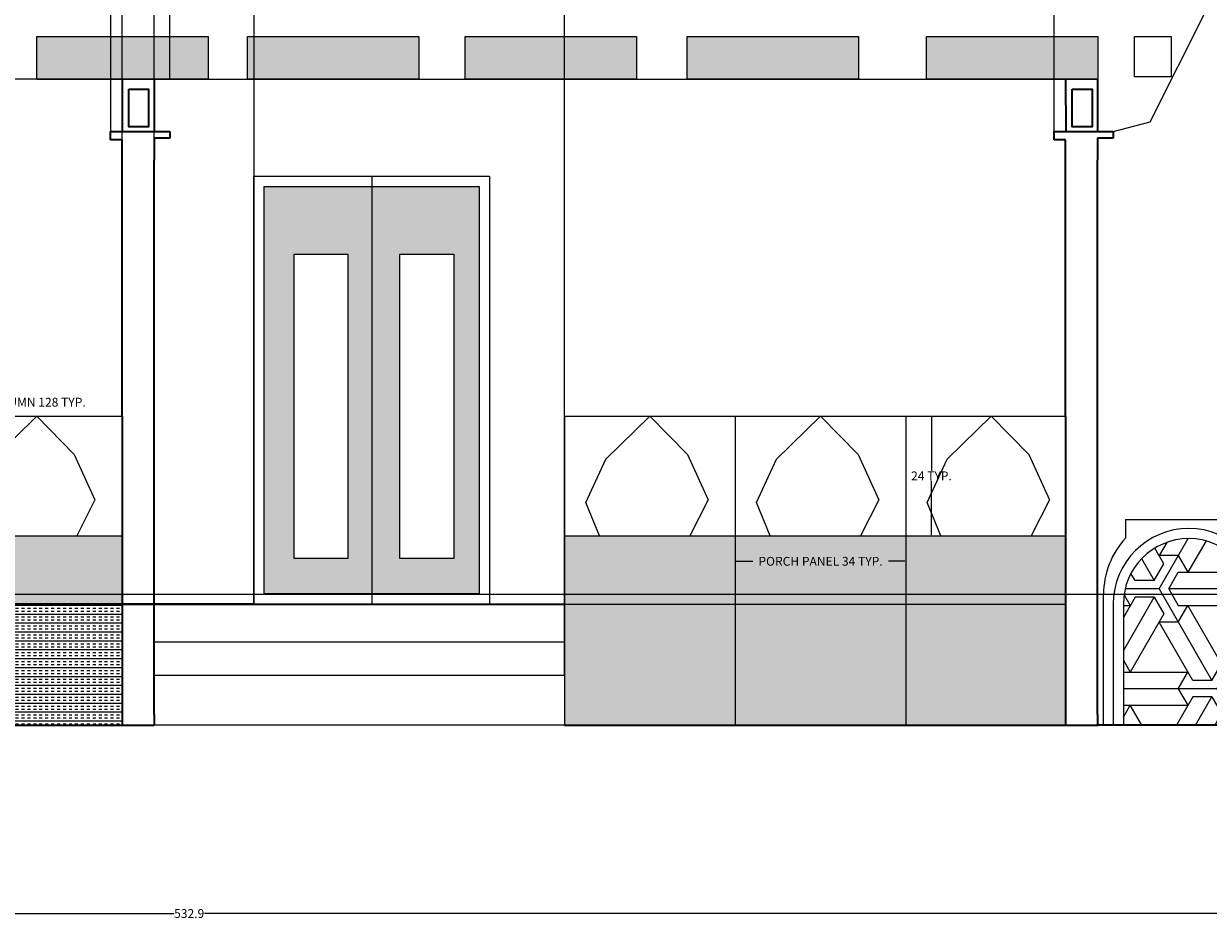
# Model space of a CAD drawing. Units: inches. Extents: x -17 to 741, y 7 to 490.
# Tile 3 of 8: x 254 to 489, y 14 to 191. Entities that reach past the tile are written whole.
import ezdxf

# ---------------------------------------------------------------- set-up
doc = ezdxf.new("R2010")
doc.units = ezdxf.units.IN
doc.header["$MEASUREMENT"] = 0
for name, color, linetype, lineweight in [('A-ANNO-DIMS', 2, 'Continuous', 18), ('A-COLS', 1, 'Continuous', 35), ('A-DOOR', 3, 'Continuous', 25), ('A-ELEV-PATT', 252, 'Continuous', 13), ('A-FLOR-RAIL', 7, 'Continuous', 25), ('A-FLOR-STRS', 7, 'Continuous', 25), ('A-ROOF-CNPE', 7, 'Continuous', 25), ('A-WALL', 7, 'Continuous', 35), ('A-WALL-PATT', 8, 'Continuous', 13), ('A-WALL-SCRN', 7, 'Continuous', 25)]:
    doc.layers.add(name, color=color, linetype=linetype, lineweight=lineweight)
doc.styles.get("Standard").update_dxf_attribs({"font": 'arial.ttf'})
doc.dimstyles.get("Standard").update_dxf_attribs({"dimtxt": 1.75, "dimasz": 0.18, "dimexe": 0.18, "dimexo": 0.0625, "dimgap": 0.09, "dimtad": 0, "dimtih": 1, "dimtoh": 1, "dimdec": 4, "dimzin": 0, "dimdsep": 46, "dimlunit": 4, "dimtxsty": 'Standard', "dimcen": 0.09, "dimadec": 0, "dimazin": 0, "dimtfac": 1, "dimtdec": 4, "dimtofl": 0, "dimtmove": 0, "dimatfit": 3, "dimfxl": 1, "dimtolj": 1, "dimtzin": 0, "dimarcsym": 0})

# ---------------------------------------------------------------- blocks, each defined once
blk = doc.blocks.new('SCREEN-ARCH-END-BAY')
for p, q in [((4.33, 40.71), (4.33, 37.01)), ((4.33, 40.71), (31.23, 40.71)), ((31.23, 40.71), (31.23, 37.52)), ((31.23, 37.52), (33.14, 37.52)), ((33.14, 37.52), (33.61, 37.52)), ((33.61, 37.52), (33.61, 0)), ((36.63, 37.52), (36.63, 0)), ((0, 0), (0, 25.9))]:
    blk.add_line(p, q)
for points in [[(31.83, 0), (31.83, 24, 1), (1.92, 24), (1.92, 0)], [(29.83, 0), (29.83, 24, 1), (3.92, 24), (3.92, 0)]]:
    blk.add_lwpolyline(points, format="xyb")
for centre, radius, start in [((35.12, 37.52), 1.51, 0), ((16.41, 25.9), 16.41, 137.3839)]:
    blk.add_arc(centre, radius, start, 180)
blk = doc.blocks.new('COL-PORCH-CAPPED')
for p, q in [((2.37, 117.52), (2.32, 127.86)), ((8.64, 117.52), (8.64, 127.86)), ((0, 115.82), (0, 117.52)), ((0, 117.52), (11.68, 117.52)), ((11.68, 117.52), (11.68, 116.2)), ((2.25, 115.82), (0, 115.82)), ((2.25, 109.13), (2.25, 115.82)), ((11.68, 116.2), (8.61, 116.2)), ((8.61, 116.2), (8.61, 111.83)), ((8.61, 2.12), (8.61, 111.83)), ((2.25, 61.18), (2.25, 109.13)), ((2.25, 61.18), (2.25, 0)), ((8.61, 2.12), (8.61, 0))]:
    blk.add_line(p, q)
blk.add_lwpolyline([(3.57, 125.89), (7.5, 125.89), (7.5, 118.41), (3.57, 118.41)], close=True)
blk = doc.blocks.new('DOOR-PAIR-FRAME')
blk.add_line((23.28, 84.63), (23.28, 0))
for points in [[(0, 84.63), (46.56, 84.63), (46.56, 0), (0, 0)], [(2, 82.63), (44.56, 82.63), (44.56, 2), (2, 2)]]:
    blk.add_lwpolyline(points, close=True)
blk = doc.blocks.new('PORCH-POINTED-PANEL')
for p, q in [((0, 23.66), (33.75, 23.66)), ((0, 0), (33.75, 0))]:
    blk.add_line(p, q)
blk.add_lwpolyline([(6.92, 0), (4.23, 6.56), (8.17, 15.14), (16.88, 23.66), (24.3, 16.07), (28.38, 7.1), (24.8, 0)])
blk = doc.blocks.new('*D17')
at = {"layer": 'A-ANNO-DIMS', "color": 0, "lineweight": -2, "transparency": 16777216}
for p, q in [((394.98, 89.46), (394.98, 84.28)), ((428.73, 89.46), (428.73, 84.28)), ((395.16, 84.46), (398.44, 84.46)), ((428.55, 84.46), (425.26, 84.46))]:
    blk.add_line(p, q, dxfattribs=at)
at = {"layer": 'A-ANNO-DIMS', "color": 0, "transparency": 16777216}
for points in [[(395.16, 84.49), (395.16, 84.43), (394.98, 84.46)], [(428.55, 84.49), (428.55, 84.43), (428.73, 84.46)]]:
    blk.add_solid(points, dxfattribs=at)
at = {"layer": 'Defpoints', "color": 0, "transparency": 16777216}
for p in [(394.98, 89.53), (428.73, 89.53), (428.73, 84.46)]:
    blk.add_point(p, dxfattribs=at)
at = {"layer": 'A-ANNO-DIMS', "color": 0, "transparency": 16777216, "insert": (411.85, 84.46), "char_height": 1.75, "attachment_point": 5}
blk.add_mtext('\\A1;PORCH PANEL 34 TYP.', dxfattribs=at)
blk = doc.blocks.new('*D18')
at = {"layer": 'A-ANNO-DIMS', "color": 0, "lineweight": -2, "transparency": 16777216}
for p, q in [((428.79, 113.19), (433.97, 113.19)), ((433.79, 113.01), (433.79, 102.33)), ((433.79, 89.71), (433.79, 100.39)), ((428.79, 89.53), (433.97, 89.53))]:
    blk.add_line(p, q, dxfattribs=at)
at = {"layer": 'A-ANNO-DIMS', "color": 0, "transparency": 16777216}
for points in [[(433.76, 113.01), (433.82, 113.01), (433.79, 113.19)], [(433.76, 89.71), (433.82, 89.71), (433.79, 89.53)]]:
    blk.add_solid(points, dxfattribs=at)
at = {"layer": 'Defpoints', "color": 0, "transparency": 16777216}
for p in [(428.73, 113.19), (433.79, 113.19), (428.73, 89.53)]:
    blk.add_point(p, dxfattribs=at)
at = {"layer": 'A-ANNO-DIMS', "color": 0, "transparency": 16777216, "insert": (433.79, 101.36), "char_height": 1.75, "attachment_point": 5}
blk.add_mtext('\\A1;24 TYP.', dxfattribs=at)
blk = doc.blocks.new('*D27')
at = {"layer": 'A-ANNO-DIMS', "color": 0, "lineweight": -2, "transparency": 16777216}
for p, q in [((271.37, 179.87), (252.08, 179.87)), ((252.26, 179.69), (252.26, 116.93)), ((252.26, 52.19), (252.26, 114.94)), ((271.37, 52.01), (252.08, 52.01))]:
    blk.add_line(p, q, dxfattribs=at)
at = {"layer": 'A-ANNO-DIMS', "color": 0, "transparency": 16777216}
for points in [[(252.23, 179.69), (252.29, 179.69), (252.26, 179.87)], [(252.23, 52.19), (252.29, 52.19), (252.26, 52.01)]]:
    blk.add_solid(points, dxfattribs=at)
at = {"layer": 'Defpoints', "color": 0, "transparency": 16777216}
for p in [(252.26, 179.87), (271.44, 179.87), (271.44, 52.01)]:
    blk.add_point(p, dxfattribs=at)
at = {"layer": 'A-ANNO-DIMS', "color": 0, "transparency": 16777216, "insert": (252.26, 115.94), "char_height": 1.75, "attachment_point": 5}
blk.add_mtext('\\A1;PORCH COLUMN 128 TYP.', dxfattribs=at)
blk = doc.blocks.new('*D28')
at = {"layer": 'A-ANNO-DIMS', "color": 0, "lineweight": -2, "transparency": 16777216}
for p, q in [((271.44, 179.93), (271.44, 199.23)), ((283.11, 179.93), (283.11, 199.23)), ((271.62, 199.05), (273.01, 199.05)), ((282.93, 199.05), (281.54, 199.05))]:
    blk.add_line(p, q, dxfattribs=at)
at = {"layer": 'A-ANNO-DIMS', "color": 0, "transparency": 16777216}
for points in [[(271.62, 199.08), (271.62, 199.02), (271.44, 199.05)], [(282.93, 199.08), (282.93, 199.02), (283.11, 199.05)]]:
    blk.add_solid(points, dxfattribs=at)
at = {"layer": 'Defpoints', "color": 0, "transparency": 16777216}
for p in [(283.11, 199.05), (271.44, 179.87), (283.11, 179.87)]:
    blk.add_point(p, dxfattribs=at)
at = {"layer": 'A-ANNO-DIMS', "color": 0, "transparency": 16777216, "insert": (277.28, 199.05), "char_height": 1.75, "attachment_point": 5}
blk.add_mtext('\\A1;12 TYP.', dxfattribs=at)
blk = doc.blocks.new('*D37')
at = {"layer": 'A-ANNO-DIMS', "color": 0, "lineweight": -2, "transparency": 16777216}
for p, q in [((20.52, 396.95), (20.52, 14.58)), ((553.43, 51.95), (553.43, 14.58)), ((20.7, 14.76), (283.93, 14.76)), ((553.25, 14.76), (290.02, 14.76))]:
    blk.add_line(p, q, dxfattribs=at)
at = {"layer": 'A-ANNO-DIMS', "color": 0, "transparency": 16777216}
for points in [[(20.7, 14.79), (20.7, 14.73), (20.52, 14.76)], [(553.25, 14.79), (553.25, 14.73), (553.43, 14.76)]]:
    blk.add_solid(points, dxfattribs=at)
at = {"layer": 'Defpoints', "color": 0, "transparency": 16777216}
for p in [(20.52, 397.01), (553.43, 52.01), (553.43, 14.76)]:
    blk.add_point(p, dxfattribs=at)
at = {"layer": 'A-ANNO-DIMS', "color": 0, "transparency": 16777216, "insert": (286.97, 14.76), "char_height": 1.75, "attachment_point": 5}
blk.add_mtext('\\A1;532.9', dxfattribs=at)
blk = doc.blocks.new('*D38')
at = {"layer": 'A-ANNO-DIMS', "color": 0, "lineweight": -2, "transparency": 16777216}
for p, q in [((341.83, 454.57), (723.06, 454.57)), ((722.88, 454.39), (722.88, 254.27)), ((722.88, 52.19), (722.88, 252.31)), ((553.49, 52.01), (723.06, 52.01))]:
    blk.add_line(p, q, dxfattribs=at)
at = {"layer": 'A-ANNO-DIMS', "color": 0, "transparency": 16777216}
for points in [[(722.85, 454.39), (722.91, 454.39), (722.88, 454.57)], [(722.85, 52.19), (722.91, 52.19), (722.88, 52.01)]]:
    blk.add_solid(points, dxfattribs=at)
at = {"layer": 'Defpoints', "color": 0, "transparency": 16777216}
for p in [(341.77, 454.57), (722.88, 454.57), (553.43, 52.01)]:
    blk.add_point(p, dxfattribs=at)
at = {"layer": 'A-ANNO-DIMS', "color": 0, "transparency": 16777216, "insert": (722.88, 253.29), "char_height": 1.75, "attachment_point": 5}
blk.add_mtext('\\A1;402.6', dxfattribs=at)
blk = doc.blocks.new('*D52')
at = {"layer": 'A-ANNO-DIMS', "color": 0, "lineweight": -2, "transparency": 16777216}
for p, q in [((239.94, 113.25), (239.94, 488.55)), ((240.12, 488.37), (253.76, 488.37)), ((273.51, 488.37), (259.86, 488.37)), ((273.69, 113.25), (273.69, 488.55))]:
    blk.add_line(p, q, dxfattribs=at)
at = {"layer": 'A-ANNO-DIMS', "color": 0, "transparency": 16777216}
for points in [[(240.12, 488.4), (240.12, 488.34), (239.94, 488.37)], [(273.51, 488.4), (273.51, 488.34), (273.69, 488.37)]]:
    blk.add_solid(points, dxfattribs=at)
at = {"layer": 'Defpoints', "color": 0, "transparency": 16777216}
for p in [(273.69, 488.37), (239.94, 113.19), (273.69, 113.19)]:
    blk.add_point(p, dxfattribs=at)
at = {"layer": 'A-ANNO-DIMS', "color": 0, "transparency": 16777216, "insert": (256.81, 488.37), "char_height": 1.75, "attachment_point": 5}
blk.add_mtext('\\A1;33.75', dxfattribs=at)
blk = doc.blocks.new('*D53')
at = {"layer": 'A-ANNO-DIMS', "color": 0, "lineweight": -2, "transparency": 16777216}
for p, q in [((271.44, 167.89), (271.44, 488.55)), ((271.62, 488.37), (361.78, 488.37)), ((457.87, 488.37), (367.7, 488.37)), ((458.05, 167.89), (458.05, 488.55))]:
    blk.add_line(p, q, dxfattribs=at)
at = {"layer": 'A-ANNO-DIMS', "color": 0, "transparency": 16777216}
for points in [[(271.62, 488.4), (271.62, 488.34), (271.44, 488.37)], [(457.87, 488.4), (457.87, 488.34), (458.05, 488.37)]]:
    blk.add_solid(points, dxfattribs=at)
at = {"layer": 'Defpoints', "color": 0, "transparency": 16777216}
for p in [(458.05, 488.37), (271.44, 167.83), (458.05, 167.83)]:
    blk.add_point(p, dxfattribs=at)
at = {"layer": 'A-ANNO-DIMS', "color": 0, "transparency": 16777216, "insert": (364.74, 488.37), "char_height": 1.75, "attachment_point": 5}
blk.add_mtext('\\A1;186.6', dxfattribs=at)
blk = doc.blocks.new('*D54')
at = {"layer": 'A-ANNO-DIMS', "color": 0, "lineweight": -2, "transparency": 16777216}
for p, q in [((458.05, 167.89), (458.05, 488.55)), ((458.23, 488.37), (502.69, 488.37)), ((553.25, 488.37), (508.78, 488.37)), ((553.43, 52.07), (553.43, 488.55))]:
    blk.add_line(p, q, dxfattribs=at)
at = {"layer": 'A-ANNO-DIMS', "color": 0, "transparency": 16777216}
for points in [[(458.23, 488.4), (458.23, 488.34), (458.05, 488.37)], [(553.25, 488.4), (553.25, 488.34), (553.43, 488.37)]]:
    blk.add_solid(points, dxfattribs=at)
at = {"layer": 'Defpoints', "color": 0, "transparency": 16777216}
for p in [(553.43, 488.37), (458.05, 167.83), (553.43, 52.01)]:
    blk.add_point(p, dxfattribs=at)
at = {"layer": 'A-ANNO-DIMS', "color": 0, "transparency": 16777216, "insert": (505.74, 488.37), "char_height": 1.75, "attachment_point": 5}
blk.add_mtext('\\A1;95.38', dxfattribs=at)
blk = doc.blocks.new('*D60')
at = {"layer": 'A-ANNO-DIMS', "color": 0, "lineweight": -2, "transparency": 16777216}
for p, q in [((280.05, 68.56), (280.05, 488.55)), ((280.23, 488.37), (286.96, 488.37)), ((299.61, 488.37), (292.87, 488.37)), ((299.79, 76.07), (299.79, 488.55))]:
    blk.add_line(p, q, dxfattribs=at)
at = {"layer": 'A-ANNO-DIMS', "color": 0, "transparency": 16777216}
for points in [[(280.23, 488.4), (280.23, 488.34), (280.05, 488.37)], [(299.61, 488.4), (299.61, 488.34), (299.79, 488.37)]]:
    blk.add_solid(points, dxfattribs=at)
at = {"layer": 'Defpoints', "color": 0, "transparency": 16777216}
for p in [(299.79, 488.37), (299.79, 76.01), (280.05, 68.49)]:
    blk.add_point(p, dxfattribs=at)
at = {"layer": 'A-ANNO-DIMS', "color": 0, "transparency": 16777216, "insert": (289.92, 488.37), "char_height": 1.75, "attachment_point": 5}
blk.add_mtext('\\A1;19.74', dxfattribs=at)
blk = doc.blocks.new('*D61')
at = {"layer": 'A-ANNO-DIMS', "color": 0, "lineweight": -2, "transparency": 16777216}
for p, q in [((225.78, 99.68), (-13.46, 99.68)), ((-13.28, 99.5), (-13.28, 88.83)), ((-13.28, 76.19), (-13.28, 86.86)), ((299.72, 76.01), (-13.46, 76.01))]:
    blk.add_line(p, q, dxfattribs=at)
at = {"layer": 'A-ANNO-DIMS', "color": 0, "transparency": 16777216}
for points in [[(-13.31, 99.5), (-13.25, 99.5), (-13.28, 99.68)], [(-13.31, 76.19), (-13.25, 76.19), (-13.28, 76.01)]]:
    blk.add_solid(points, dxfattribs=at)
at = {"layer": 'Defpoints', "color": 0, "transparency": 16777216}
for p in [(225.85, 99.68), (-13.28, 76.01), (299.79, 76.01)]:
    blk.add_point(p, dxfattribs=at)
at = {"layer": 'A-ANNO-DIMS', "color": 0, "transparency": 16777216, "insert": (-13.28, 87.85), "char_height": 1.75, "attachment_point": 5}
blk.add_mtext('\\A1;23.677', dxfattribs=at)
blk = doc.blocks.new('*D64')
at = {"layer": 'A-ANNO-DIMS', "color": 0, "lineweight": -2, "transparency": 16777216}
for p, q in [((516.74, 77.91), (-13.46, 77.91)), ((-13.28, 77.73), (-13.28, 65.94)), ((-13.28, 52.19), (-13.28, 63.98)), ((516.74, 52.01), (-13.46, 52.01))]:
    blk.add_line(p, q, dxfattribs=at)
at = {"layer": 'A-ANNO-DIMS', "color": 0, "transparency": 16777216}
for points in [[(-13.31, 77.73), (-13.25, 77.73), (-13.28, 77.91)], [(-13.31, 52.19), (-13.25, 52.19), (-13.28, 52.01)]]:
    blk.add_solid(points, dxfattribs=at)
at = {"layer": 'Defpoints', "color": 0, "transparency": 16777216}
for p in [(-13.28, 77.91), (516.8, 77.91), (516.8, 52.01)]:
    blk.add_point(p, dxfattribs=at)
at = {"layer": 'A-ANNO-DIMS', "color": 0, "transparency": 16777216, "insert": (-13.28, 64.96), "char_height": 1.75, "attachment_point": 5}
blk.add_mtext('\\A1;25.9', dxfattribs=at)
blk = doc.blocks.new('*D68')
at = {"layer": 'A-ANNO-DIMS', "color": 0, "lineweight": -2, "transparency": 16777216}
for p, q in [((280.05, 61.98), (280.05, 488.55)), ((280.23, 488.37), (317.59, 488.37)), ((361.04, 488.37), (323.68, 488.37)), ((361.22, 61.98), (361.22, 488.55))]:
    blk.add_line(p, q, dxfattribs=at)
at = {"layer": 'A-ANNO-DIMS', "color": 0, "transparency": 16777216}
for points in [[(280.23, 488.4), (280.23, 488.34), (280.05, 488.37)], [(361.04, 488.4), (361.04, 488.34), (361.22, 488.37)]]:
    blk.add_solid(points, dxfattribs=at)
at = {"layer": 'Defpoints', "color": 0, "transparency": 16777216}
for p in [(361.22, 488.37), (280.05, 61.91), (361.22, 61.91)]:
    blk.add_point(p, dxfattribs=at)
at = {"layer": 'A-ANNO-DIMS', "color": 0, "transparency": 16777216, "insert": (320.64, 488.37), "char_height": 1.75, "attachment_point": 5}
blk.add_mtext('\\A1;81.18', dxfattribs=at)

msp = doc.modelspace()

# ---------------------------------------------------------------- hatches: boundary and pattern name
at = {"layer": 'A-ELEV-PATT'}
h = msp.add_hatch(dxfattribs=at)
h.set_pattern_fill('STARS', color=256, scale=19)
h.paths.add_polyline_path([(204.6793, 330.2905), (174.1219, 330.2905), (174.1219, 324.7204), (204.6793, 324.7204)])
h.paths.add_polyline_path([(238.7618, 330.6251), (208.2044, 330.6251), (208.2044, 325.055), (238.7618, 325.055)])
h.paths.add_polyline_path([(316.4391, 354.2167), (282.5434, 354.2167), (282.5434, 345.7496), (316.4391, 345.7496)])
h.paths.add_polyline_path([(360.3395, 354.2167), (326.4438, 354.2167), (326.4438, 345.7496), (360.3395, 345.7496)])
h.paths.add_polyline_path([(407.6938, 354.2167), (373.7981, 354.2167), (373.7981, 345.7496), (407.6938, 345.7496)])
h.paths.add_polyline_path([(290.7055, 188.3373), (256.8098, 188.3373), (256.8098, 179.8702), (290.7055, 179.8702)])
h.paths.add_polyline_path([(332.372, 188.3373), (298.4763, 188.3373), (298.4763, 179.8702), (332.372, 179.8702)])
h.paths.add_polyline_path([(375.4339, 188.3373), (341.5382, 188.3373), (341.5382, 179.8702), (375.4339, 179.8702)])
h.paths.add_polyline_path([(419.3343, 188.3373), (385.4386, 188.3373), (385.4386, 179.8702), (419.3343, 179.8702)])
h.paths.add_polyline_path([(466.6886, 188.3373), (432.7929, 188.3373), (432.7929, 179.8702), (466.6886, 179.8702)])
h = msp.add_hatch(color=256, dxfattribs=at)
h.dxf.hatch_style = 1
h.paths.add_polyline_path([(323.0665, 158.6389), (301.7867, 158.6389), (301.7867, 78.0082), (323.0665, 78.0082)])
h.paths.add_polyline_path([(318.3825, 145.2592), (318.3825, 85.0354), (307.7462, 85.0354), (307.7462, 145.2592)], flags=16)
h.paths.add_polyline_path([(344.3462, 158.6389), (323.0665, 158.6389), (323.0665, 78.0082), (344.3462, 78.0082)])
h.paths.add_polyline_path([(339.3004, 145.2592), (339.3004, 85.0354), (328.6642, 85.0354), (328.6642, 145.2592)], flags=16)
h.paths.add_polyline_path([(192.7233, 151.6028), (190.2672, 151.6028), (190.2672, 142.0361), (192.7233, 142.0361)])
h.paths.add_polyline_path([(192.7233, 141.0361), (190.2672, 141.0361), (190.2672, 135.6738), (192.7233, 135.6738)])
h.paths.add_polyline_path([(192.7233, 142.0361), (190.2672, 142.0361), (190.2672, 141.0361), (192.7233, 141.0361)])
h.paths.add_polyline_path([(209.3698, 142.0361), (192.7233, 142.0361), (192.7233, 141.0361), (209.3698, 141.0361)])
h.paths.add_polyline_path([(190.2672, 142.0361), (183.5379, 142.0361), (183.5379, 141.0361), (190.2672, 141.0361)])
h.paths.add_polyline_path([(190.2672, 135.6738), (183.5379, 135.6738), (183.5379, 134.6738), (190.2672, 134.6738)])
h.paths.add_polyline_path([(192.7233, 135.6738), (190.2672, 135.6738), (190.2672, 134.6738), (192.7233, 134.6738)])
h.paths.add_polyline_path([(192.7233, 134.6738), (190.2672, 134.6738), (190.2672, 101.6848), (192.7233, 101.6848)])
h.paths.add_polyline_path([(209.3698, 135.6738), (192.7233, 135.6738), (192.7233, 134.6738), (209.3698, 134.6738)])
h.paths.add_polyline_path([(211.8259, 135.6738), (209.3698, 135.6738), (209.3698, 134.6738), (211.8259, 134.6738)])
h.paths.add_polyline_path([(211.8259, 141.0361), (209.3698, 141.0361), (209.3698, 135.6738), (211.8259, 135.6738)])
h.paths.add_polyline_path([(211.8259, 142.0361), (209.3698, 142.0361), (209.3698, 141.0361), (211.8259, 141.0361)])
h.paths.add_polyline_path([(211.8259, 151.6028), (209.3698, 151.6028), (209.3698, 142.0361), (211.8259, 142.0361)])
h.paths.add_polyline_path([(223.8474, 142.0361), (211.8259, 142.0361), (211.8259, 141.0361), (223.8474, 141.0361)])
h.paths.add_polyline_path([(223.8474, 135.6738), (211.8259, 135.6738), (211.8259, 134.6738), (223.8474, 134.6738)])
h.paths.add_polyline_path([(211.8259, 134.6738), (209.3698, 134.6738), (209.3698, 108.8153), (211.8259, 108.8153)])
h.paths.add_polyline_path([(211.8259, 108.8153), (209.3698, 108.8153), (209.3698, 107.8153), (211.8259, 107.8153)])
h.paths.add_polyline_path([(211.8259, 107.8153), (209.3698, 107.8153), (209.3698, 101.6848), (211.8259, 101.6848)])
h.paths.add_polyline_path([(223.8474, 108.8153), (211.8259, 108.8153), (211.8259, 107.8153), (223.8474, 107.8153)])
h.paths.add_polyline_path([(209.3698, 108.8153), (192.7233, 108.8153), (192.7233, 107.8153), (209.3698, 107.8153)])
h.paths.add_polyline_path([(190.2672, 108.8153), (183.5379, 108.8153), (183.5379, 107.8153), (190.2672, 107.8153)])
h.paths.add_polyline_path([(147.2864, 151.6028), (144.8304, 151.6028), (144.8304, 109.315), (147.2864, 109.315)])
h.paths.add_polyline_path([(147.2864, 109.315), (144.8304, 109.315), (144.8304, 108.315), (147.2864, 108.315)])
h.paths.add_polyline_path([(147.2864, 108.315), (144.8304, 108.315), (144.8304, 101.6848), (147.2864, 101.6848)])
h.paths.add_polyline_path([(157.8499, 109.315), (147.2864, 109.315), (147.2864, 108.315), (157.8499, 108.315)])
h.paths.add_polyline_path([(144.8304, 109.315), (127.7745, 109.315), (127.7745, 108.315), (144.8304, 108.315)])
h.paths.add_polyline_path([(127.7745, 109.315), (125.3184, 109.315), (125.3184, 108.315), (127.7745, 108.315)])
h.paths.add_polyline_path([(127.7745, 151.6028), (125.3184, 151.6028), (125.3184, 109.315), (127.7745, 109.315)])
h.paths.add_polyline_path([(125.3184, 109.315), (117.5405, 109.315), (117.5405, 108.315), (125.3184, 108.315)])
h.paths.add_polyline_path([(127.7745, 108.315), (125.3184, 108.315), (125.3184, 101.6848), (127.7745, 101.6848)])
h.paths.add_polyline_path([(125.3184, 135.9009), (117.5405, 135.9009), (117.5405, 134.9009), (125.3184, 134.9009)])
h.paths.add_polyline_path([(144.8304, 135.9009), (127.7745, 135.9009), (127.7745, 134.9009), (144.8304, 134.9009)])
h.paths.add_polyline_path([(157.8499, 135.9009), (147.2864, 135.9009), (147.2864, 134.9009), (157.8499, 134.9009)])
h.paths.add_polyline_path([(144.8304, 142.0361), (127.7745, 142.0361), (127.7745, 141.0361), (144.8304, 141.0361)])
h.paths.add_polyline_path([(157.8499, 142.0361), (147.2864, 142.0361), (147.2864, 141.0361), (157.8499, 141.0361)])
h.paths.add_polyline_path([(125.3184, 142.0361), (117.5405, 142.0361), (117.5405, 141.0361), (125.3184, 141.0361)])
h.paths.add_polyline_path([(447.5234, 311.9659), (445.0673, 311.9659), (445.0673, 302.3991), (447.5234, 302.3991)])
h.paths.add_polyline_path([(447.5234, 302.3991), (445.0673, 302.3991), (445.0673, 301.3991), (447.5234, 301.3991)])
h.paths.add_polyline_path([(458.0869, 302.3991), (447.5234, 302.3991), (447.5234, 301.3991), (458.0869, 301.3991)])
h.paths.add_polyline_path([(447.5234, 301.3991), (445.0673, 301.3991), (445.0673, 296.2639), (447.5234, 296.2639)])
h.paths.add_polyline_path([(447.5234, 296.2639), (445.0673, 296.2639), (445.0673, 295.2639), (447.5234, 295.2639)])
h.paths.add_polyline_path([(458.0869, 296.2639), (447.5234, 296.2639), (447.5234, 295.2639), (458.0869, 295.2639)])
h.paths.add_polyline_path([(445.0673, 296.2639), (428.0115, 296.2639), (428.0115, 295.2639), (445.0673, 295.2639)])
h.paths.add_polyline_path([(447.5234, 295.2639), (445.0673, 295.2639), (445.0673, 262.0479), (447.5234, 262.0479)])
h.paths.add_polyline_path([(445.0673, 302.3991), (428.0115, 302.3991), (428.0115, 301.3991), (445.0673, 301.3991)])
h.paths.add_polyline_path([(428.0115, 302.3991), (425.5554, 302.3991), (425.5554, 301.3991), (428.0115, 301.3991)])
h.paths.add_polyline_path([(428.0115, 311.9659), (425.5554, 311.9659), (425.5554, 302.3991), (428.0115, 302.3991)])
h.paths.add_polyline_path([(425.5554, 302.3991), (417.7774, 302.3991), (417.7774, 301.3991), (425.5554, 301.3991)])
h.paths.add_polyline_path([(428.0115, 301.3991), (425.5554, 301.3991), (425.5554, 296.2639), (428.0115, 296.2639)])
h.paths.add_polyline_path([(425.5554, 296.2639), (417.7774, 296.2639), (417.7774, 295.2639), (425.5554, 295.2639)])
h.paths.add_polyline_path([(428.0115, 296.2639), (425.5554, 296.2639), (425.5554, 295.2639), (428.0115, 295.2639)])
h.paths.add_polyline_path([(428.0115, 295.2639), (425.5554, 295.2639), (425.5554, 262.0479), (428.0115, 262.0479)])
h.paths.add_polyline_path([(425.5554, 269.8939), (417.7774, 269.8939), (417.7774, 268.8939), (425.5554, 268.8939)])
h.paths.add_polyline_path([(445.0673, 269.8939), (428.0115, 269.8939), (428.0115, 268.8939), (445.0673, 268.8939)])
h.paths.add_polyline_path([(458.0869, 269.8939), (447.5234, 269.8939), (447.5234, 268.8939), (458.0869, 268.8939)])
at = {"layer": 'A-WALL-PATT'}
h = msp.add_hatch(dxfattribs=at)
h.set_pattern_fill('EARTH', color=256, scale=13, angle=16)
h.paths.add_polyline_path([(273.6893, 89.5255), (239.9367, 89.5255), (239.9367, 76.0082), (273.6893, 76.0082)])
h.paths.add_polyline_path([(394.976, 89.5255), (361.2234, 89.5255), (361.2234, 76.0082), (394.976, 76.0082)])
h.paths.add_polyline_path([(428.7285, 89.5255), (394.976, 89.5255), (394.976, 76.0082), (428.7285, 76.0082)])
h.paths.add_polyline_path([(460.302, 89.5255), (428.7285, 89.5255), (428.7285, 76.0082), (460.302, 76.0082)])
h.paths.add_polyline_path([(239.9367, 220.0082), (98.075, 220.0082), (98.075, 212.3604), (237.0146, 212.3604)])
h = msp.add_hatch(dxfattribs=at)
h.set_pattern_fill('ESCHER', color=256, scale=19)
h.paths.add_polyline_path([(497.6481, 76.0082, 1), (471.7452, 76.0082), (471.7452, 52.0082), (497.6481, 52.0082)])
h.paths.add_polyline_path([(546.6242, 76.0082, 1), (520.7212, 76.0082), (520.7212, 52.0082), (546.6242, 52.0082)])
h = msp.add_hatch(dxfattribs=at)
h.set_pattern_fill('INSUL', color=256, scale=4.7)
h.paths.add_polyline_path([(273.6893, 76.0082), (239.9367, 76.0082), (239.9367, 52.0082), (273.6893, 52.0082)])
h = msp.add_hatch(dxfattribs=at)
h.set_pattern_fill('INSUL', color=256, scale=4.7)
h.paths.add_polyline_path([(394.976, 76.0082), (361.2234, 76.0082), (361.2234, 52.0082), (394.976, 52.0082)])
h.paths.add_polyline_path([(428.7285, 76.0082), (394.976, 76.0082), (394.976, 52.0082), (428.7285, 52.0082)])
h.paths.add_polyline_path([(460.302, 76.0082), (428.7285, 76.0082), (428.7285, 52.0082), (460.302, 52.0082)])

# ---------------------------------------------------------------- linework, layer by layer
at = {"layer": 'A-DOOR'}
for points in [[(307.7462, 145.2592), (318.3825, 145.2592), (318.3825, 85.0354), (307.7462, 85.0354)], [(328.6642, 145.2592), (339.3004, 145.2592), (339.3004, 85.0354), (328.6642, 85.0354)]]:
    msp.add_lwpolyline(points, close=True, dxfattribs=at)
at = {"layer": 'A-FLOR-RAIL'}
for p, q in [((361.2234, 113.1863), (361.2234, 76.0082)), ((394.976, 113.1863), (394.976, 52.0082)), ((428.7285, 113.1863), (428.7285, 52.0082)), ((428.7285, 113.1863), (460.302, 113.1863)), ((428.7285, 89.5255), (460.302, 89.5255)), ((361.2234, 76.0082), (361.2234, 52.0082)), ((361.2234, 76.0082), (460.302, 76.0082))]:
    msp.add_line(p, q, dxfattribs=at)
msp.add_lwpolyline([(435.6456, 89.5255), (432.9627, 96.0908), (436.8976, 104.6692), (445.6048, 113.1863), (453.0329, 105.5924), (457.1087, 96.6269), (453.5316, 89.5255)], dxfattribs=at)
at = {"layer": 'A-FLOR-STRS'}
for p, q in [((280.0481, 68.493), (361.2234, 68.493)), ((280.0481, 61.9147), (361.2234, 61.9147))]:
    msp.add_line(p, q, dxfattribs=at)
at = {"layer": 'A-ROOF-CNPE'}
msp.add_line((256.8098, 179.8702), (466.6886, 179.8702), dxfattribs=at)
msp.add_lwpolyline([(469.6986, 169.533), (477.0431, 171.3989), (488.0578, 193.3539)], dxfattribs=at)
for points in [[(256.8098, 188.3373), (290.7055, 188.3373), (290.7055, 179.8702), (256.8098, 179.8702)], [(298.4763, 188.3373), (332.372, 188.3373), (332.372, 179.8702), (298.4763, 179.8702)], [(341.5382, 188.3373), (375.4339, 188.3373), (375.4339, 179.8702), (341.5382, 179.8702)], [(385.4386, 188.3373), (419.3343, 188.3373), (419.3343, 179.8702), (385.4386, 179.8702)], [(432.7929, 188.3373), (466.6886, 188.3373), (466.6886, 179.8702), (432.7929, 179.8702)], [(473.9821, 188.3373), (481.1765, 188.3373), (481.1765, 180.2979), (473.9821, 180.2979)]]:
    msp.add_lwpolyline(points, close=True, dxfattribs=at)
at = {"layer": 'A-WALL'}
for p, q in [((53.4591, 76.0082), (361.2234, 76.0082)), ((53.4591, 52.0082), (280.0481, 52.0082)), ((361.2234, 52.0082), (466.6607, 52.0082)), ((553.4286, 52.0082), (466.6607, 52.0082))]:
    msp.add_line(p, q, dxfattribs=at)

# ---------------------------------------------------------------- block references
at = {"layer": 'A-COLS'}
for p in [(271.437, 52.008), (458.0497, 52.008)]:
    msp.add_blockref('COL-PORCH-CAPPED', p, dxfattribs=at)
at = {"layer": 'A-DOOR'}
msp.add_blockref('DOOR-PAIR-FRAME', (299.787, 76.008), dxfattribs=at)
at = {"layer": 'A-FLOR-RAIL'}
for p in [(239.937, 89.526), (361.2237, 89.526), (394.9762, 89.526)]:
    msp.add_blockref('PORCH-POINTED-PANEL', p, dxfattribs=at)
at = {"layer": 'A-WALL-SCRN'}
msp.add_blockref('SCREEN-ARCH-END-BAY', (467.8218, 52.008), dxfattribs=at)

# ---------------------------------------------------------------- dimensions: what is measured, and where the dimension line sits
at = {"layer": 'A-ANNO-DIMS'}
for base, p1, p2, override, picture, middle in [((273.6893, 488.3717), (239.9367, 113.1863), (273.6893, 113.1863), {"dimdec": 2, "dimlfac": 1, "dimrnd": 0, "dimzin": 0, "dimdsep": 46, "dimlunit": 2}, '*D52', (256.813, 488.3717)), ((458.0494, 488.3717), (271.4367, 167.8255), (458.0494, 167.8255), {"dimdec": 1, "dimlfac": 1, "dimrnd": 0, "dimzin": 0, "dimdsep": 46, "dimlunit": 2}, '*D53', (364.743, 488.3717)), ((299.7867, 488.3717), (280.0481, 68.493), (299.7867, 76.0082), {"dimdec": 2, "dimlfac": 1, "dimrnd": 0, "dimzin": 0, "dimdsep": 46, "dimlunit": 2}, '*D60', (289.9174, 488.3717)), ((361.2234, 488.3717), (280.0481, 61.9147), (361.2234, 61.9147), {"dimdec": 2, "dimlfac": 1, "dimrnd": 0, "dimzin": 0, "dimdsep": 46, "dimlunit": 2}, '*D68', (320.6357, 488.3717)), ((553.4286, 488.3717), (458.0494, 167.8255), (553.4286, 52.0082), {"dimdec": 2, "dimlfac": 1, "dimrnd": 0, "dimzin": 0, "dimdsep": 46, "dimlunit": 2}, '*D54', (505.739, 488.3717)), ((553.4286, 14.7597), (20.5169, 397.0087), (553.4286, 52.0082), {"dimdec": 1, "dimlfac": 1, "dimrnd": 0, "dimzin": 0, "dimdsep": 46, "dimlunit": 2}, '*D37', (286.9727, 14.7597))]:
    dim = msp.add_linear_dim(base=base, p1=p1, p2=p2, dimstyle='Standard', override=override, dxfattribs=at)
    dim.commit()
    dim.dimension.update_dxf_attribs({"geometry": picture, "text_midpoint": middle})
for base, p1, p2, override, picture, middle in [((722.8826, 454.5717), (553.4286, 52.0082), (341.7687, 454.5717), {"dimdec": 1, "dimlfac": 1, "dimrnd": 0, "dimzin": 0, "dimdsep": 46, "dimlunit": 2}, '*D38', (722.8826, 253.2899)), ((-13.2831, 76.0082), (225.8474, 99.6848), (299.7867, 76.0082), {"dimdec": 3, "dimlfac": 1, "dimrnd": 0, "dimzin": 0, "dimdsep": 46, "dimlunit": 2}, '*D61', (-13.2831, 87.8465)), ((-13.2831, 77.9092), (516.7979, 52.0082), (516.7979, 77.9092), {"dimdec": 1, "dimlfac": 1, "dimrnd": 0, "dimzin": 0, "dimdsep": 46, "dimlunit": 2}, '*D64', (-13.2831, 64.9587))]:
    dim = msp.add_linear_dim(base=base, p1=p1, p2=p2, angle=90, dimstyle='Standard', override=override, dxfattribs=at)
    dim.commit()
    dim.dimension.update_dxf_attribs({"geometry": picture, "text_midpoint": middle})
for base, p1, p2, text, picture, middle in [((283.1138, 199.0495), (271.4367, 179.8702), (283.1138, 179.8702), '<> TYP.', '*D28', (277.2752, 199.0495)), ((428.7285, 84.4626), (394.976, 89.5255), (428.7285, 89.5255), 'PORCH PANEL <> TYP.', '*D17', (411.8523, 84.4626))]:
    dim = msp.add_linear_dim(base=base, p1=p1, p2=p2, text=text, dimstyle='Standard', override={"dimdec": 0, "dimlfac": 1, "dimrnd": 0, "dimzin": 0, "dimdsep": 46, "dimlunit": 2}, dxfattribs=at)
    dim.commit()
    dim.dimension.update_dxf_attribs({"geometry": picture, "text_midpoint": middle})
for base, p1, p2, text, picture, middle in [((252.2574, 179.8702), (271.4367, 52.0082), (271.4367, 179.8702), 'PORCH COLUMN <> TYP.', '*D27', (252.2574, 115.9392)), ((433.7914, 113.1863), (428.7285, 89.5255), (428.7285, 113.1863), '<> TYP.', '*D18', (433.7914, 101.3559))]:
    dim = msp.add_linear_dim(base=base, p1=p1, p2=p2, angle=90, text=text, dimstyle='Standard', override={"dimdec": 0, "dimlfac": 1, "dimrnd": 0, "dimzin": 0, "dimdsep": 46, "dimlunit": 2}, dxfattribs=at)
    dim.commit()
    dim.dimension.update_dxf_attribs({"geometry": picture, "text_midpoint": middle})

doc.saveas('drawing.dxf')
